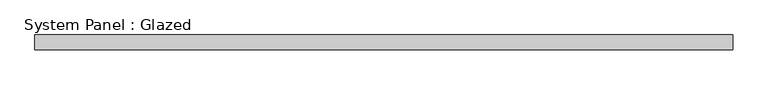
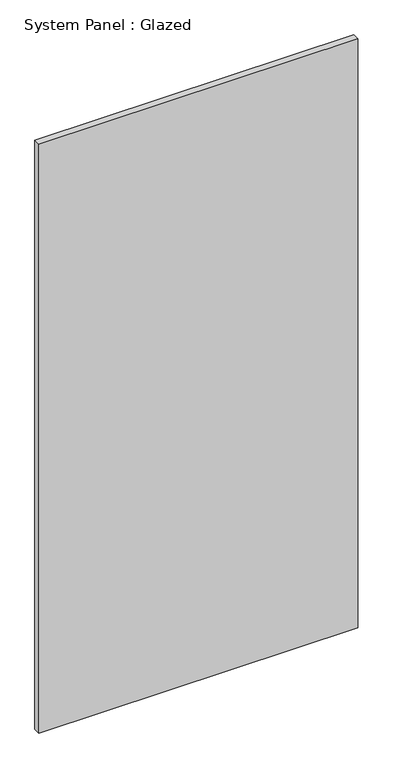
"""IFC4 building model written with IfcOpenShell, lengths in millimetres: plate geometry, System Panel : Glazed."""

from ifc_helpers import new_model, si_unit, origin, origin_with_axes, place, context, project, spatial, polyline, outline, extrude, source, transform, mapped, element, save


def system_panel_glazed_33731b62(model_context):
    return source(origin(), model_context, "Body", "SweptSolid", [
        extrude(outline(polyline([(600.0750001, 19.05), (-600.0750001, 19.05), (-600.0750001, 44.45), (600.0750001, 44.45), (600.0750001, 19.05)])), origin_with_axes(), (0.0, 0.0, 1.0), 2343.15),
    ])


if __name__ == "__main__":
    model = new_model("IFC4")
    model_context = context("Model", 3, world=origin())
    ifc_project = project(units=[si_unit("LENGTHUNIT", "METRE", prefix="MILLI")], contexts=[model_context])
    site = spatial("IfcSite", under=ifc_project)
    building = spatial("IfcBuilding", under=site)
    placement = place(None, origin())
    system_panel_glazed_shape = system_panel_glazed_33731b62(model_context)
    element("IfcPlate", 1, ObjectType="System Panel : Glazed", at=placement, inside=building, context=model_context, shape_type="MappedRepresentation", body=[
        mapped(system_panel_glazed_shape, transform((0.0, 0.0, 0.0), x_axis=(1.0, 0.0, 0.0), y_axis=(0.0, 1.0, 0.0), z_axis=(0.0, 0.0, 1.0))),
    ])
    save(model, "model.ifc")

# Revit data of these elements
# Type "System Panel : Glazed"
#   Construction Type Id = "GSP4R"
#   Analytic Construction = "1/8 in Pilkington single glazing"
#   Visual Light Transmittance = 0.9
#   Solar Heat Gain Coefficient = 0.86
#   Heat Transfer Coefficient (U) = 1.18115 BTU/(h·ft²·°F)
#   Define Thermal Properties by = 1
# Element 1 (IfcPlate, "System Panel : Glazed")
#   Materials on its faces: "Glass"
# Materials
#   "Glass": class "Glass", colour RGB 0 128 192, transparency 0.75, Description = "Soda Lime Glass", Cost = 0
